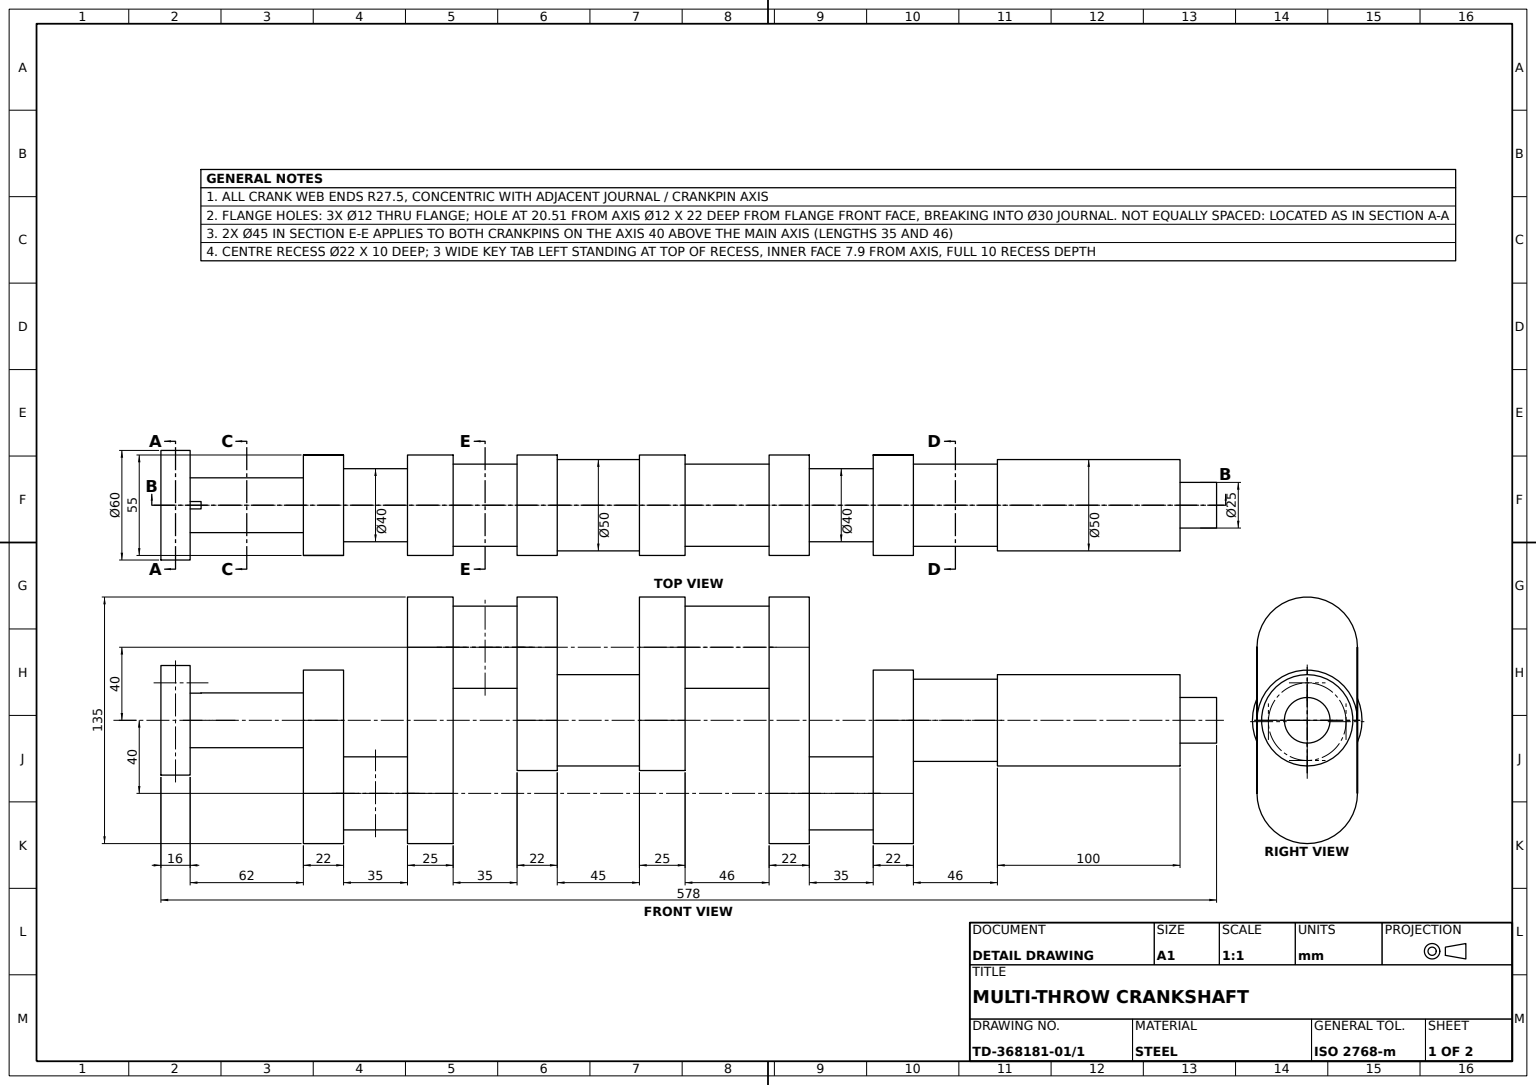
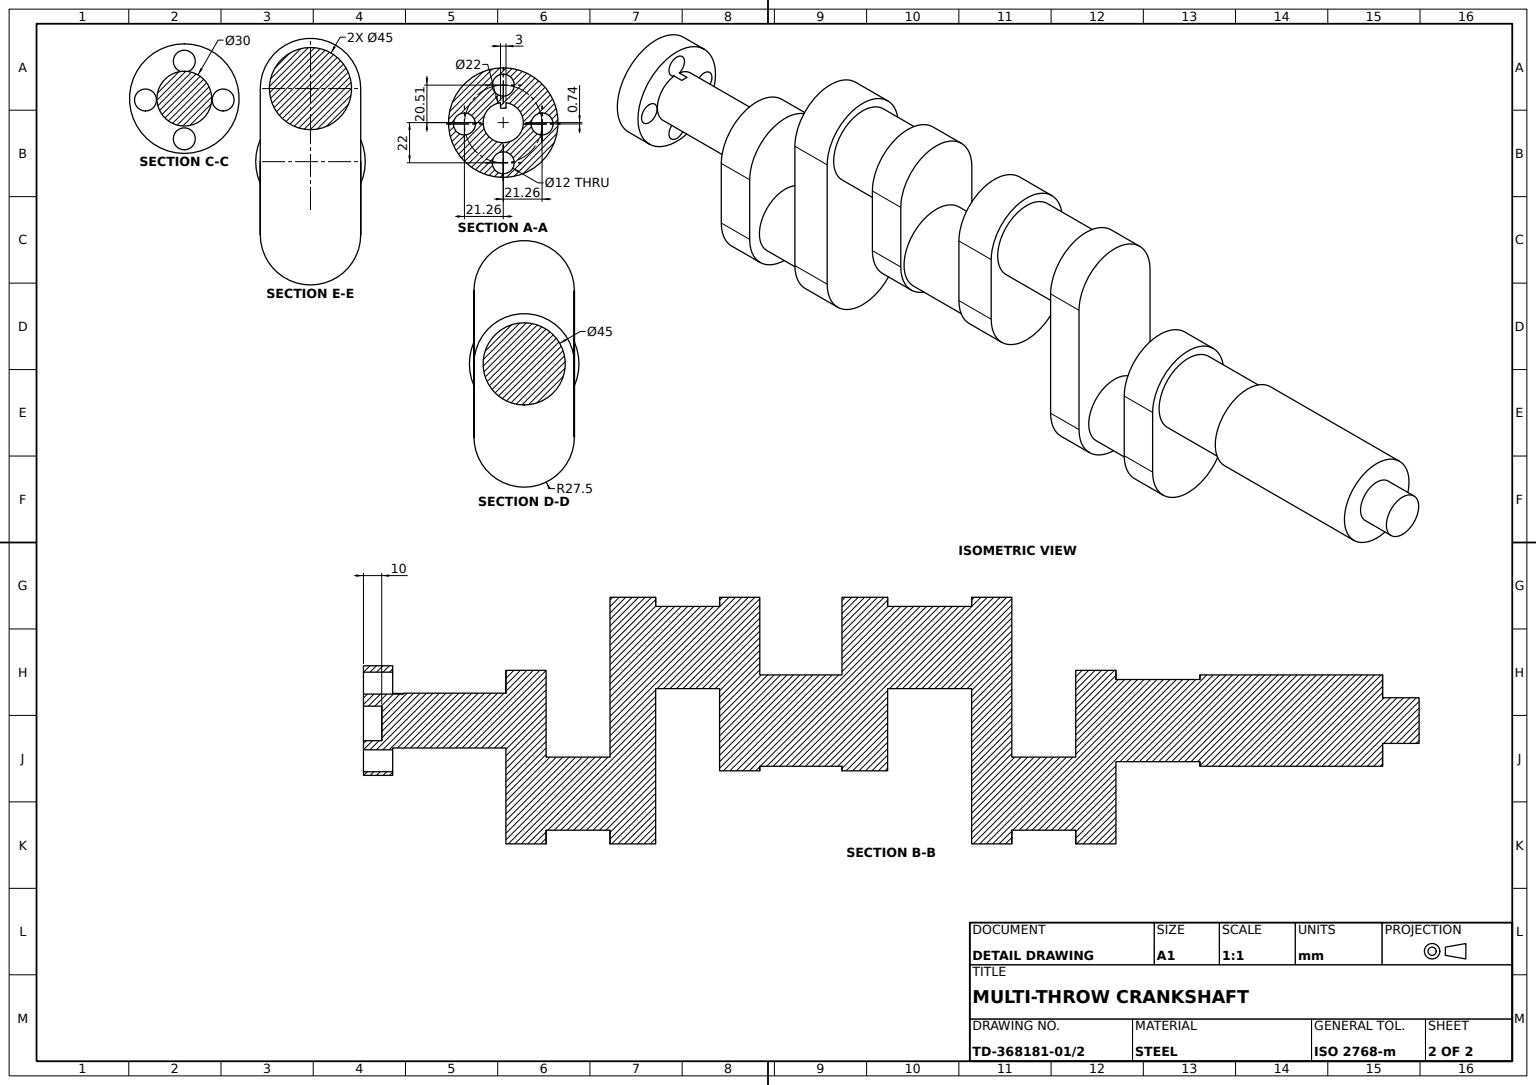
from build123d import *

# Parameters (mm, degrees)
FLANGE_SKETCH_R              = 30
FRONT_FLANGE_60_DEPTH        = 16
FRONT_MAIN_JOURNAL_PROFILE_W = 15
FRONT_MAIN_JOURNAL_PROFILE_H = 62
CRANK_WEB_1_DEPTH            = 22
CRANKPIN_1_PROFILE_W         = 20
CRANKPIN_1_PROFILE_H         = 35
CRANK_WEB_2_DEPTH            = 25
MAIN_JOURNAL_2_PROFILE_W     = 22.5
MAIN_JOURNAL_2_PROFILE_H     = 35
CRANK_WEB_3_DEPTH            = 22
CRANKPIN_2_PROFILE_W         = 25
CRANKPIN_2_PROFILE_H         = 45
CRANK_WEB_4_DEPTH            = 25
MAIN_JOURNAL_3_PROFILE_W     = 22.5
MAIN_JOURNAL_3_PROFILE_H     = 46
CRANK_WEB_5_DEPTH            = 22
CRANKPIN_3_PROFILE_W         = 20
CRANKPIN_3_PROFILE_H         = 35
CRANK_WEB_6_SKETCH_R         = 20
CRANK_WEB_6_DEPTH            = 22
REAR_MAIN_JOURNAL_PROFILE_W  = 22.5
REAR_MAIN_JOURNAL_PROFILE_H  = 46
OUTPUT_SHAFT_PROFILE_W       = 25
OUTPUT_SHAFT_PROFILE_H       = 100
END_SPIGOT_PROFILE_W         = 12.5
END_SPIGOT_PROFILE_H         = 20
FLANGE_BOLT_HOLES_SKETCH_R   = 6
FLANGE_BOLT_HOLES_4X_DEPTH   = 22
FLANGE_CENTRE_RECESS_DEPTH   = 10


with BuildPart() as part:
    # Flange Sketch → Front Flange _60 (new body)
    with BuildSketch(Plane.XY):
        Circle(FLANGE_SKETCH_R)
    extrude(amount=FRONT_FLANGE_60_DEPTH)

    # Front Main Journal Profile → Front Main Journal (revolve)
    with BuildSketch(Plane(origin=(0, 0, 0), x_dir=(1, 0, 0), z_dir=(0, 1, 0)), mode=Mode.PRIVATE) as front_main_journal_sk:
        with Locations((7.5, 31)):
            Rectangle(FRONT_MAIN_JOURNAL_PROFILE_W, FRONT_MAIN_JOURNAL_PROFILE_H)
    revolve(front_main_journal_sk.sketch.rotate(Axis((0, 0, -63.530762812), (0, 0, 1)), 180), axis=Axis((0, 0, -63.530762812), (0, 0, 1)))

    # Crank Web 1 Sketch → Crank Web 1 (add)
    with BuildSketch(Plane(origin=(0, 0, -62), x_dir=(-1, 0, 0), z_dir=(0, 0, -1))):
        with BuildLine():
            Line((-40, 27.5), (0, 27.5))
            ThreePointArc((0, 27.5), (27.5, 0), (0, -27.5))
            Line((0, -27.5), (-40, -27.5))
            ThreePointArc((-40, -27.5), (-67.5, 0), (-40, 27.5))
        make_face()
    extrude(amount=CRANK_WEB_1_DEPTH)

    # Crankpin 1 Profile → Crankpin 1 (revolve)
    with BuildSketch(Plane(origin=(0, 0, 0), x_dir=(1, 0, 0), z_dir=(0, 1, 0))):
        with Locations((50, 101.5)):
            Rectangle(CRANKPIN_1_PROFILE_W, CRANKPIN_1_PROFILE_H)
    revolve(axis=Axis((40, 0, -84), (0, 0, -1)))

    # Crank Web 2 Sketch → Crank Web 2 (add)
    with BuildSketch(Plane(origin=(0, 0, -119), x_dir=(-1, 0, 0), z_dir=(0, 0, -1))):
        with BuildLine():
            Line((-40, 27.5), (40, 27.5))
            ThreePointArc((40, 27.5), (67.5, 0), (40, -27.5))
            Line((40, -27.5), (-40, -27.5))
            ThreePointArc((-40, -27.5), (-67.5, 0), (-40, 27.5))
        make_face()
    extrude(amount=CRANK_WEB_2_DEPTH)

    # Main Journal 2 Profile → Main Journal 2 (revolve)
    with BuildSketch(Plane(origin=(0, 0, 0), x_dir=(1, 0, 0), z_dir=(0, 1, 0))):
        with Locations((-28.75, 161.5)):
            Rectangle(MAIN_JOURNAL_2_PROFILE_W, MAIN_JOURNAL_2_PROFILE_H)
    revolve(axis=Axis((-40, 0, -144), (0, 0, -1)))

    # Crank Web 3 Sketch → Crank Web 3 (add)
    with BuildSketch(Plane(origin=(0, 0, -179), x_dir=(-1, 0, 0), z_dir=(0, 0, -1))):
        with BuildLine():
            Line((0, 27.5), (40, 27.5))
            ThreePointArc((40, 27.5), (67.5, 0), (40, -27.5))
            Line((40, -27.5), (0, -27.5))
            ThreePointArc((0, -27.5), (-27.5, 0), (0, 27.5))
        make_face()
    extrude(amount=CRANK_WEB_3_DEPTH)

    # Crankpin 2 Profile → Crankpin 2 (revolve)
    with BuildSketch(Plane(origin=(0, 0, 0), x_dir=(1, 0, 0), z_dir=(0, 1, 0)), mode=Mode.PRIVATE) as crankpin_2_sk:
        with Locations((12.5, 223.5)):
            Rectangle(CRANKPIN_2_PROFILE_W, CRANKPIN_2_PROFILE_H)
    revolve(crankpin_2_sk.sketch.rotate(Axis((0, 0, -261.148585065), (0, 0, 1)), 180), axis=Axis((0, 0, -261.148585065), (0, 0, 1)))

    # Crank Web 4 Sketch → Crank Web 4 (add)
    with BuildSketch(Plane(origin=(0, 0, -246), x_dir=(-1, 0, 0), z_dir=(0, 0, -1))):
        with BuildLine():
            Line((0, 27.5), (40, 27.5))
            ThreePointArc((40, 27.5), (67.5, 0), (40, -27.5))
            Line((40, -27.5), (0, -27.5))
            ThreePointArc((0, -27.5), (-27.5, 0), (0, 27.5))
        make_face()
    extrude(amount=CRANK_WEB_4_DEPTH)

    # Main Journal 3 Profile → Main Journal 3 (revolve)
    with BuildSketch(Plane(origin=(0, 0, 0), x_dir=(1, 0, 0), z_dir=(0, 1, 0))):
        with Locations((-28.75, 294)):
            Rectangle(MAIN_JOURNAL_3_PROFILE_W, MAIN_JOURNAL_3_PROFILE_H)
    revolve(axis=Axis((-40, 0, -271), (0, 0, -1)))

    # Crank Web 5 Sketch → Crank Web 5 (add)
    with BuildSketch(Plane(origin=(0, 0, -317), x_dir=(-1, 0, 0), z_dir=(0, 0, -1))):
        with BuildLine():
            Line((-40, 27.5), (40, 27.5))
            ThreePointArc((40, 27.5), (67.5, 0), (40, -27.5))
            Line((40, -27.5), (-40, -27.5))
            ThreePointArc((-40, -27.5), (-67.5, 0), (-40, 27.5))
        make_face()
    extrude(amount=CRANK_WEB_5_DEPTH)

    # Crankpin 3 Profile → Crankpin 3 (revolve)
    with BuildSketch(Plane(origin=(0, 0, 0), x_dir=(1, 0, 0), z_dir=(0, 1, 0))):
        with Locations((50, 356.5)):
            Rectangle(CRANKPIN_3_PROFILE_W, CRANKPIN_3_PROFILE_H)
    revolve(axis=Axis((40, 0, -339), (0, 0, -1)))

    # Crank Web 6 Sketch → Crank Web 6 (add)
    # profile 1 of 2: a face of its own
    with BuildSketch(Plane(origin=(0, 0, -374), x_dir=(-1, 0, 0), z_dir=(0, 0, -1))):
        with BuildLine():
            Line((-40, -27.5), (0, -27.5))
            ThreePointArc((0, -27.5), (27.5, 0), (0, 27.5))
            Line((0, 27.5), (-40, 27.5))
            ThreePointArc((-40, 27.5), (-67.5, 0), (-40, -27.5))
        make_face()
        with Locations(Location((-40, 0, 0), (0, 0, 180))):
            Circle(CRANK_WEB_6_SKETCH_R, mode=Mode.SUBTRACT)
    # profile 2 of 2: a face of its own
    with BuildSketch(Plane(origin=(0, 0, -374), x_dir=(-1, 0, 0), z_dir=(0, 0, -1))):
        with Locations(Location((-40, 0, 0), (0, 0, 180))):
            Circle(CRANK_WEB_6_SKETCH_R)
    extrude(amount=CRANK_WEB_6_DEPTH)

    # Rear Main Journal Profile → Rear Main Journal (revolve)
    with BuildSketch(Plane(origin=(0, 0, 0), x_dir=(1, 0, 0), z_dir=(0, 1, 0))):
        with Locations((11.25, 419)):
            Rectangle(REAR_MAIN_JOURNAL_PROFILE_W, REAR_MAIN_JOURNAL_PROFILE_H)
    revolve(axis=Axis((0, 0, -396), (0, 0, -1)))

    # Output Shaft Profile → Output Shaft (revolve)
    with BuildSketch(Plane(origin=(0, 0, 0), x_dir=(1, 0, 0), z_dir=(0, 1, 0))):
        with Locations((12.5, 492)):
            Rectangle(OUTPUT_SHAFT_PROFILE_W, OUTPUT_SHAFT_PROFILE_H)
    revolve(axis=Axis((0, 0, -442), (0, 0, -1)))

    # End Spigot Profile → End Spigot (revolve)
    with BuildSketch(Plane(origin=(0, 0, 0), x_dir=(1, 0, 0), z_dir=(0, 1, 0))):
        with Locations((6.25, 552)):
            Rectangle(END_SPIGOT_PROFILE_W, END_SPIGOT_PROFILE_H)
    revolve(axis=Axis((0, 0, -542), (0, 0, -1)))

    # Flange Bolt Holes Sketch → Flange Bolt Holes 4x (cut)
    with BuildSketch(Plane.XY.offset(16)):
        with Locations((22, 0)):
            Circle(FLANGE_BOLT_HOLES_SKETCH_R)
        with Locations((0.74374517, -21.25625483)):
            Circle(FLANGE_BOLT_HOLES_SKETCH_R)
        with Locations((-20.512509661, 0)):
            Circle(FLANGE_BOLT_HOLES_SKETCH_R)
        with Locations((0.74374517, 21.25625483)):
            Circle(FLANGE_BOLT_HOLES_SKETCH_R)
    extrude(amount=-FLANGE_BOLT_HOLES_4X_DEPTH, mode=Mode.SUBTRACT)

    # Flange Centre Recess Sketch → Flange Centre Recess (cut)
    with BuildSketch(Plane.XY.offset(16)):
        with BuildLine():
            Line((-10.897247359, 1.5), (-7.897247359, 1.5))
            Line((-7.897247359, 1.5), (-7.897247359, -1.5))
            Line((-7.897247359, -1.5), (-10.897247359, -1.5))
            ThreePointArc((-10.897247359, -1.5), (11, 0), (-10.897247359, 1.5))
        make_face()
    extrude(amount=-FLANGE_CENTRE_RECESS_DEPTH, mode=Mode.SUBTRACT)


solid = part.part
